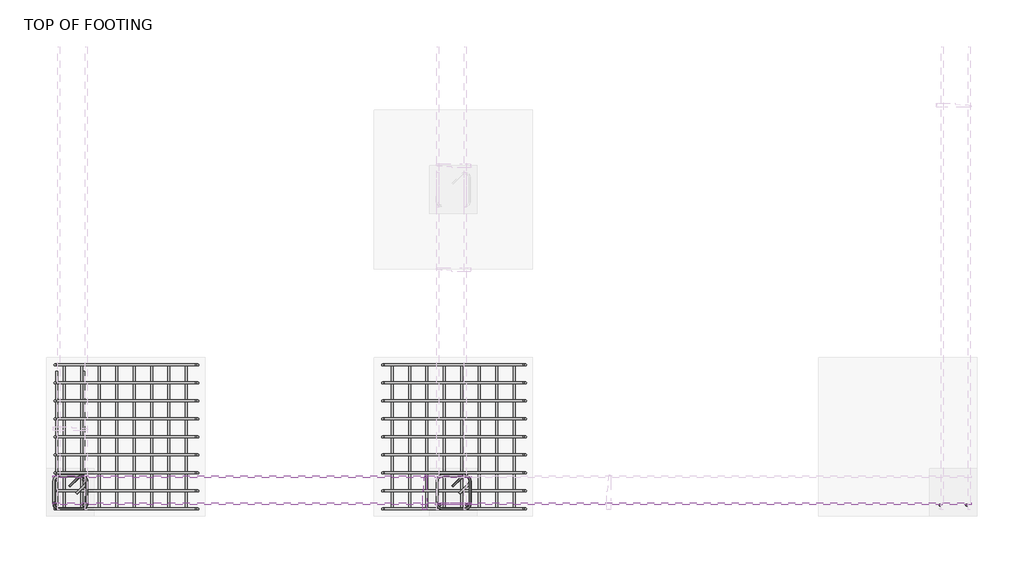
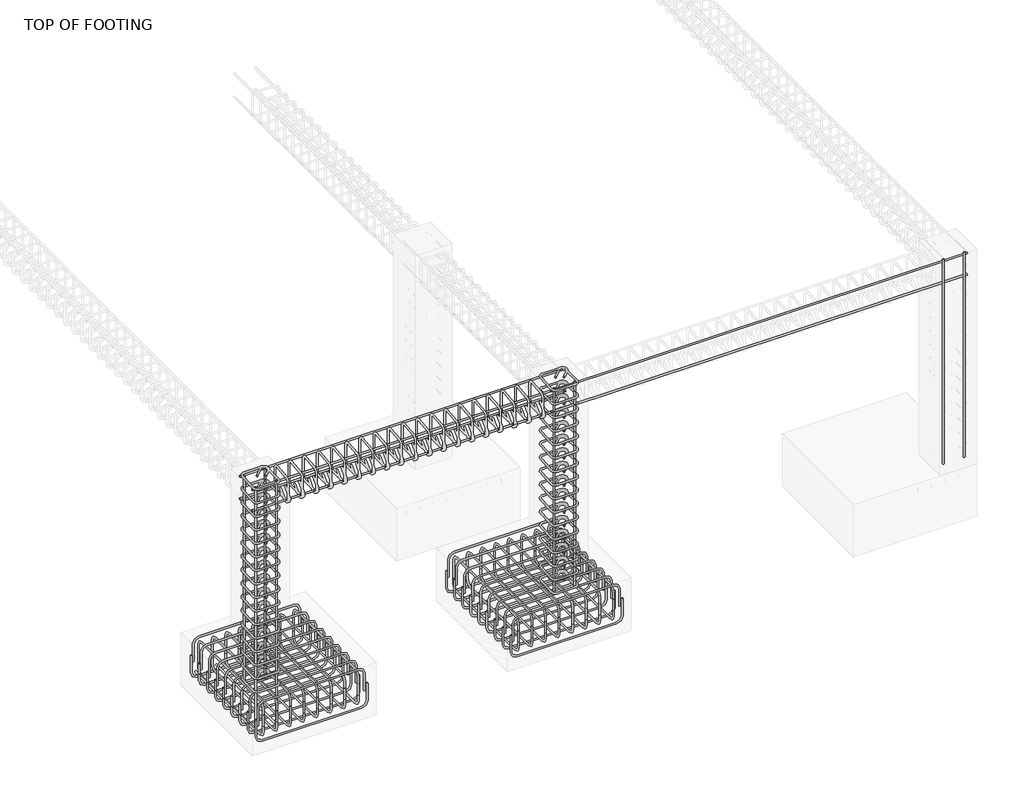
# One storey, part 2 of 10: 18 reinforcing bars.
"""IFC4 building model written with IfcOpenShell, lengths in millimetres."""

from ifc_helpers import new_model, si_unit, point, frame, origin, place, context, project, spatial, polyline, circle_curve, trimmed, segment, composite_curve, source, transform, mapped, element, save
from ifc_brep_helpers import swept_disk

model = new_model("IFC4")

# Units and contexts
model_context = context("Model", 3, world=origin())
ifc_project = project(units=[si_unit("LENGTHUNIT", "METRE", prefix="MILLI")], contexts=[model_context])

# Site, building, storey
site = spatial("IfcSite", under=ifc_project)
building = spatial("IfcBuilding", under=site)
storey = spatial("IfcBuildingStorey", under=building, Name="TOP OF FOOTING", Elevation=-1828.8)

# Reinforcing bars
placement = place(None, origin())
reinforcing_bar_shape = source(origin(), model_context, "Body", "SolidModel", [
    swept_disk(composite_curve([segment(polyline([(-9737.3957678, 8861.0767485, -2013.6880036), (-9737.3957678, 8861.0767485, -2160.9880036)]), True, "CONTINUOUS"), segment(trimmed(circle_curve(frame((-9783.7457678, 8861.0767485, -2160.9880036), z_axis=(0.0, 1.0, 0.0), x_axis=(46.349999999998545, 0.0, 0.0)), 46.35), [point((-9737.3957678, 8861.0767485, -2160.9880036))], [point((-9783.7457678, 8861.0767485, -2207.3380036))], True, "CARTESIAN"), True, "CONTINUOUS"), segment(polyline([(-9783.7457678, 8861.0767485, -2207.3380036), (-10591.4530437, 8861.0767485, -2207.3380036)]), True, "CONTINUOUS"), segment(trimmed(circle_curve(frame((-10591.4530437, 8861.0767485, -2160.9880036), z_axis=(0.0, 1.0, 0.0), x_axis=(0.0, 0.0, -46.34999999999991)), 46.35), [point((-10591.4530437, 8861.0767485, -2207.3380036))], [point((-10637.8030437, 8861.0767485, -2160.9880036))], True, "CARTESIAN"), True, "CONTINUOUS"), segment(polyline([(-10637.8030437, 8861.0767485, -2160.9880036), (-10637.8030437, 8861.0767485, -2013.6880036)]), True, "CONTINUOUS")], self_intersect=False), 6.35),
])
element("IfcReinforcingBar", 1, at=placement, inside=storey, context=model_context, shape_type="MappedRepresentation", body=[
    mapped(reinforcing_bar_shape, transform((0.0, 0.0, 0.0), x_axis=(1.0, 0.0, 0.0), y_axis=(0.0, 1.0, 0.0), z_axis=(0.0, 0.0, 1.0))),
    mapped(reinforcing_bar_shape, transform((0.0, -113.4125, 0.0), x_axis=(1.0, 0.0, 0.0), y_axis=(0.0, 1.0, 0.0), z_axis=(0.0, 0.0, 1.0))),
    mapped(reinforcing_bar_shape, transform((0.0, -226.825, 0.0), x_axis=(1.0, 0.0, 0.0), y_axis=(0.0, 1.0, 0.0), z_axis=(0.0, 0.0, 1.0))),
    mapped(reinforcing_bar_shape, transform((0.0, -340.2375, 0.0), x_axis=(1.0, 0.0, 0.0), y_axis=(0.0, 1.0, 0.0), z_axis=(0.0, 0.0, 1.0))),
    mapped(reinforcing_bar_shape, transform((0.0, -453.65, 0.0), x_axis=(1.0, 0.0, 0.0), y_axis=(0.0, 1.0, 0.0), z_axis=(0.0, 0.0, 1.0))),
    mapped(reinforcing_bar_shape, transform((0.0, -567.0625, 0.0), x_axis=(1.0, 0.0, 0.0), y_axis=(0.0, 1.0, 0.0), z_axis=(0.0, 0.0, 1.0))),
    mapped(reinforcing_bar_shape, transform((0.0, -680.475, 0.0), x_axis=(1.0, 0.0, 0.0), y_axis=(0.0, 1.0, 0.0), z_axis=(0.0, 0.0, 1.0))),
    mapped(reinforcing_bar_shape, transform((0.0, -793.8875, 0.0), x_axis=(1.0, 0.0, 0.0), y_axis=(0.0, 1.0, 0.0), z_axis=(0.0, 0.0, 1.0))),
    mapped(reinforcing_bar_shape, transform((0.0, -907.3, 0.0), x_axis=(1.0, 0.0, 0.0), y_axis=(0.0, 1.0, 0.0), z_axis=(0.0, 0.0, 1.0))),
])
reinforcing_bar_2_shape = source(origin(), model_context, "Body", "SolidModel", [
    swept_disk(composite_curve([segment(polyline([(-10621.5548549, 8861.0767485, -2068.7560969), (-10621.5548549, 8861.0767485, -1921.4560969)]), True, "CONTINUOUS"), segment(trimmed(circle_curve(frame((-10575.2048549, 8861.0767485, -1921.4560969), z_axis=(0.0, 1.0, 0.0), x_axis=(-46.350000000000364, 0.0, 0.0)), 46.35), [point((-10621.5548549, 8861.0767485, -1921.4560969))], [point((-10575.2048549, 8861.0767485, -1875.1060969))], True, "CARTESIAN"), True, "CONTINUOUS"), segment(polyline([(-10575.2048549, 8861.0767485, -1875.1060969), (-9806.8133686, 8861.0767485, -1875.1060969)]), True, "CONTINUOUS"), segment(trimmed(circle_curve(frame((-9806.8133686, 8861.0767485, -1921.4560969), z_axis=(0.0, 1.0, 0.0), x_axis=(0.0, 0.0, 46.34999999999991)), 46.35), [point((-9806.8133686, 8861.0767485, -1875.1060969))], [point((-9760.4633686, 8861.0767485, -1921.4560969))], True, "CARTESIAN"), True, "CONTINUOUS"), segment(polyline([(-9760.4633686, 8861.0767485, -1921.4560969), (-9760.4633686, 8861.0767485, -2068.7560969)]), True, "CONTINUOUS")], self_intersect=False), 6.35),
])
element("IfcReinforcingBar", 2, at=placement, inside=storey, context=model_context, shape_type="MappedRepresentation", body=[
    mapped(reinforcing_bar_2_shape, transform((0.0, 0.0, 0.0), x_axis=(1.0, 0.0, 0.0), y_axis=(0.0, 1.0, 0.0), z_axis=(0.0, 0.0, 1.0))),
    mapped(reinforcing_bar_2_shape, transform((0.0, -113.4125, 0.0), x_axis=(1.0, 0.0, 0.0), y_axis=(0.0, 1.0, 0.0), z_axis=(0.0, 0.0, 1.0))),
    mapped(reinforcing_bar_2_shape, transform((0.0, -226.825, 0.0), x_axis=(1.0, 0.0, 0.0), y_axis=(0.0, 1.0, 0.0), z_axis=(0.0, 0.0, 1.0))),
    mapped(reinforcing_bar_2_shape, transform((0.0, -340.2375, 0.0), x_axis=(1.0, 0.0, 0.0), y_axis=(0.0, 1.0, 0.0), z_axis=(0.0, 0.0, 1.0))),
    mapped(reinforcing_bar_2_shape, transform((0.0, -453.65, 0.0), x_axis=(1.0, 0.0, 0.0), y_axis=(0.0, 1.0, 0.0), z_axis=(0.0, 0.0, 1.0))),
    mapped(reinforcing_bar_2_shape, transform((0.0, -567.0625, 0.0), x_axis=(1.0, 0.0, 0.0), y_axis=(0.0, 1.0, 0.0), z_axis=(0.0, 0.0, 1.0))),
    mapped(reinforcing_bar_2_shape, transform((0.0, -680.475, 0.0), x_axis=(1.0, 0.0, 0.0), y_axis=(0.0, 1.0, 0.0), z_axis=(0.0, 0.0, 1.0))),
    mapped(reinforcing_bar_2_shape, transform((0.0, -793.8875, 0.0), x_axis=(1.0, 0.0, 0.0), y_axis=(0.0, 1.0, 0.0), z_axis=(0.0, 0.0, 1.0))),
    mapped(reinforcing_bar_2_shape, transform((0.0, -907.3, 0.0), x_axis=(1.0, 0.0, 0.0), y_axis=(0.0, 1.0, 0.0), z_axis=(0.0, 0.0, 1.0))),
])
reinforcing_bar_3_shape = source(origin(), model_context, "Body", "SolidModel", [
    swept_disk(composite_curve([segment(polyline([(-9809.6682872, 8861.0767485, -2087.4821199), (-9809.6682872, 8861.0767485, -1940.1821199)]), True, "CONTINUOUS"), segment(trimmed(circle_curve(frame((-9809.6682872, 8814.7267485, -1940.1821199), z_axis=(1.0, 0.0, 0.0), x_axis=(0.0, 46.350000000000364, 0.0)), 46.35), [point((-9809.6682872, 8861.0767485, -1940.1821199))], [point((-9809.6682872, 8814.7267485, -1893.8321199))], True, "CARTESIAN"), True, "CONTINUOUS"), segment(polyline([(-9809.6682872, 8814.7267485, -1893.8321199), (-9809.6682872, 8000.1267485, -1893.8321199)]), True, "CONTINUOUS"), segment(trimmed(circle_curve(frame((-9809.6682872, 8000.1267485, -1940.1821199), z_axis=(1.0, 0.0, 0.0), x_axis=(0.0, 0.0, 46.350000000000136)), 46.35), [point((-9809.6682872, 8000.1267485, -1893.8321199))], [point((-9809.6682872, 7953.7767485, -1940.1821199))], True, "CARTESIAN"), True, "CONTINUOUS"), segment(polyline([(-9809.6682872, 7953.7767485, -1940.1821199), (-9809.6682872, 7953.7767485, -2087.4821199)]), True, "CONTINUOUS")], self_intersect=False), 6.35),
])
element("IfcReinforcingBar", 3, at=placement, inside=storey, context=model_context, shape_type="MappedRepresentation", body=[
    mapped(reinforcing_bar_3_shape, transform((0.0, 0.0, 0.0), x_axis=(1.0, 0.0, 0.0), y_axis=(0.0, 1.0, 0.0), z_axis=(0.0, 0.0, 1.0))),
    mapped(reinforcing_bar_3_shape, transform((-109.824938, 0.0, 0.0), x_axis=(1.0, 0.0, 0.0), y_axis=(0.0, 1.0, 0.0), z_axis=(0.0, 0.0, 1.0))),
    mapped(reinforcing_bar_3_shape, transform((-219.649876, 0.0, 0.0), x_axis=(1.0, 0.0, 0.0), y_axis=(0.0, 1.0, 0.0), z_axis=(0.0, 0.0, 1.0))),
    mapped(reinforcing_bar_3_shape, transform((-329.474814, 0.0, 0.0), x_axis=(1.0, 0.0, 0.0), y_axis=(0.0, 1.0, 0.0), z_axis=(0.0, 0.0, 1.0))),
    mapped(reinforcing_bar_3_shape, transform((-439.299752, 0.0, 0.0), x_axis=(1.0, 0.0, 0.0), y_axis=(0.0, 1.0, 0.0), z_axis=(0.0, 0.0, 1.0))),
    mapped(reinforcing_bar_3_shape, transform((-549.12469, 0.0, 0.0), x_axis=(1.0, 0.0, 0.0), y_axis=(0.0, 1.0, 0.0), z_axis=(0.0, 0.0, 1.0))),
    mapped(reinforcing_bar_3_shape, transform((-658.949628, 0.0, 0.0), x_axis=(1.0, 0.0, 0.0), y_axis=(0.0, 1.0, 0.0), z_axis=(0.0, 0.0, 1.0))),
    mapped(reinforcing_bar_3_shape, transform((-768.774566, 0.0, 0.0), x_axis=(1.0, 0.0, 0.0), y_axis=(0.0, 1.0, 0.0), z_axis=(0.0, 0.0, 1.0))),
])
reinforcing_bar_4_shape = source(origin(), model_context, "Body", "SolidModel", [
    swept_disk(composite_curve([segment(polyline([(-10578.4428532, 8861.0767485, -1990.1985611), (-10578.4428532, 8861.0767485, -2137.4985611)]), True, "CONTINUOUS"), segment(trimmed(circle_curve(frame((-10578.4428532, 8814.7267485, -2137.4985611), z_axis=(-1.0, 0.0, 0.0), x_axis=(0.0, 46.350000000000364, 0.0)), 46.35), [point((-10578.4428532, 8861.0767485, -2137.4985611))], [point((-10578.4428532, 8814.7267485, -2183.8485611))], True, "CARTESIAN"), True, "CONTINUOUS"), segment(polyline([(-10578.4428532, 8814.7267485, -2183.8485611), (-10578.4428532, 8000.1267485, -2183.8485611)]), True, "CONTINUOUS"), segment(trimmed(circle_curve(frame((-10578.4428532, 8000.1267485, -2137.4985611), z_axis=(-1.0, 0.0, 0.0), x_axis=(0.0, 0.0, -46.34999999999991)), 46.35), [point((-10578.4428532, 8000.1267485, -2183.8485611))], [point((-10578.4428532, 7953.7767485, -2137.4985611))], True, "CARTESIAN"), True, "CONTINUOUS"), segment(polyline([(-10578.4428532, 7953.7767485, -2137.4985611), (-10578.4428532, 7953.7767485, -1990.1985611)]), True, "CONTINUOUS")], self_intersect=False), 6.35),
])
element("IfcReinforcingBar", 4, at=placement, inside=storey, context=model_context, shape_type="MappedRepresentation", body=[
    mapped(reinforcing_bar_4_shape, transform((0.0, 0.0, 0.0), x_axis=(1.0, 0.0, 0.0), y_axis=(0.0, 1.0, 0.0), z_axis=(0.0, 0.0, 1.0))),
    mapped(reinforcing_bar_4_shape, transform((109.824938, 0.0, 0.0), x_axis=(1.0, 0.0, 0.0), y_axis=(0.0, 1.0, 0.0), z_axis=(0.0, 0.0, 1.0))),
    mapped(reinforcing_bar_4_shape, transform((219.649876, 0.0, 0.0), x_axis=(1.0, 0.0, 0.0), y_axis=(0.0, 1.0, 0.0), z_axis=(0.0, 0.0, 1.0))),
    mapped(reinforcing_bar_4_shape, transform((329.474814, 0.0, 0.0), x_axis=(1.0, 0.0, 0.0), y_axis=(0.0, 1.0, 0.0), z_axis=(0.0, 0.0, 1.0))),
    mapped(reinforcing_bar_4_shape, transform((439.299752, 0.0, 0.0), x_axis=(1.0, 0.0, 0.0), y_axis=(0.0, 1.0, 0.0), z_axis=(0.0, 0.0, 1.0))),
    mapped(reinforcing_bar_4_shape, transform((549.12469, 0.0, 0.0), x_axis=(1.0, 0.0, 0.0), y_axis=(0.0, 1.0, 0.0), z_axis=(0.0, 0.0, 1.0))),
    mapped(reinforcing_bar_4_shape, transform((658.949628, 0.0, 0.0), x_axis=(1.0, 0.0, 0.0), y_axis=(0.0, 1.0, 0.0), z_axis=(0.0, 0.0, 1.0))),
    mapped(reinforcing_bar_4_shape, transform((768.774566, 0.0, 0.0), x_axis=(1.0, 0.0, 0.0), y_axis=(0.0, 1.0, 0.0), z_axis=(0.0, 0.0, 1.0))),
])
reinforcing_bar_5_shape = source(origin(), model_context, "Body", "SolidModel", [
    swept_disk(composite_curve([segment(polyline([(-7671.9957678, 8861.0767485, -2013.6880036), (-7671.9957678, 8861.0767485, -2160.9880036)]), True, "CONTINUOUS"), segment(trimmed(circle_curve(frame((-7718.3457678, 8861.0767485, -2160.9880036), z_axis=(0.0, 1.0, 0.0), x_axis=(46.350000000000364, 0.0, 0.0)), 46.35), [point((-7671.9957678, 8861.0767485, -2160.9880036))], [point((-7718.3457678, 8861.0767485, -2207.3380036))], True, "CARTESIAN"), True, "CONTINUOUS"), segment(polyline([(-7718.3457678, 8861.0767485, -2207.3380036), (-8526.0530437, 8861.0767485, -2207.3380036)]), True, "CONTINUOUS"), segment(trimmed(circle_curve(frame((-8526.0530437, 8861.0767485, -2160.9880036), z_axis=(0.0, 1.0, 0.0), x_axis=(0.0, 0.0, -46.34999999999991)), 46.35), [point((-8526.0530437, 8861.0767485, -2207.3380036))], [point((-8572.4030437, 8861.0767485, -2160.9880036))], True, "CARTESIAN"), True, "CONTINUOUS"), segment(polyline([(-8572.4030437, 8861.0767485, -2160.9880036), (-8572.4030437, 8861.0767485, -2013.6880036)]), True, "CONTINUOUS")], self_intersect=False), 6.35),
])
element("IfcReinforcingBar", 5, at=placement, inside=storey, context=model_context, shape_type="MappedRepresentation", body=[
    mapped(reinforcing_bar_5_shape, transform((0.0, 0.0, 0.0), x_axis=(1.0, 0.0, 0.0), y_axis=(0.0, 1.0, 0.0), z_axis=(0.0, 0.0, 1.0))),
    mapped(reinforcing_bar_5_shape, transform((0.0, -113.4125, 0.0), x_axis=(1.0, 0.0, 0.0), y_axis=(0.0, 1.0, 0.0), z_axis=(0.0, 0.0, 1.0))),
    mapped(reinforcing_bar_5_shape, transform((0.0, -226.825, 0.0), x_axis=(1.0, 0.0, 0.0), y_axis=(0.0, 1.0, 0.0), z_axis=(0.0, 0.0, 1.0))),
    mapped(reinforcing_bar_5_shape, transform((0.0, -340.2375, 0.0), x_axis=(1.0, 0.0, 0.0), y_axis=(0.0, 1.0, 0.0), z_axis=(0.0, 0.0, 1.0))),
    mapped(reinforcing_bar_5_shape, transform((0.0, -453.65, 0.0), x_axis=(1.0, 0.0, 0.0), y_axis=(0.0, 1.0, 0.0), z_axis=(0.0, 0.0, 1.0))),
    mapped(reinforcing_bar_5_shape, transform((0.0, -567.0625, 0.0), x_axis=(1.0, 0.0, 0.0), y_axis=(0.0, 1.0, 0.0), z_axis=(0.0, 0.0, 1.0))),
    mapped(reinforcing_bar_5_shape, transform((0.0, -680.475, 0.0), x_axis=(1.0, 0.0, 0.0), y_axis=(0.0, 1.0, 0.0), z_axis=(0.0, 0.0, 1.0))),
    mapped(reinforcing_bar_5_shape, transform((0.0, -793.8875, 0.0), x_axis=(1.0, 0.0, 0.0), y_axis=(0.0, 1.0, 0.0), z_axis=(0.0, 0.0, 1.0))),
    mapped(reinforcing_bar_5_shape, transform((0.0, -907.3, 0.0), x_axis=(1.0, 0.0, 0.0), y_axis=(0.0, 1.0, 0.0), z_axis=(0.0, 0.0, 1.0))),
])
reinforcing_bar_6_shape = source(origin(), model_context, "Body", "SolidModel", [
    swept_disk(composite_curve([segment(polyline([(-8556.1548549, 8861.0767485, -2068.7560969), (-8556.1548549, 8861.0767485, -1921.4560969)]), True, "CONTINUOUS"), segment(trimmed(circle_curve(frame((-8509.8048549, 8861.0767485, -1921.4560969), z_axis=(0.0, 1.0, 0.0), x_axis=(-46.350000000000364, 0.0, 0.0)), 46.35), [point((-8556.1548549, 8861.0767485, -1921.4560969))], [point((-8509.8048549, 8861.0767485, -1875.1060969))], True, "CARTESIAN"), True, "CONTINUOUS"), segment(polyline([(-8509.8048549, 8861.0767485, -1875.1060969), (-7741.4133686, 8861.0767485, -1875.1060969)]), True, "CONTINUOUS"), segment(trimmed(circle_curve(frame((-7741.4133686, 8861.0767485, -1921.4560969), z_axis=(0.0, 1.0, 0.0), x_axis=(0.0, 0.0, 46.34999999999991)), 46.35), [point((-7741.4133686, 8861.0767485, -1875.1060969))], [point((-7695.0633686, 8861.0767485, -1921.4560969))], True, "CARTESIAN"), True, "CONTINUOUS"), segment(polyline([(-7695.0633686, 8861.0767485, -1921.4560969), (-7695.0633686, 8861.0767485, -2068.7560969)]), True, "CONTINUOUS")], self_intersect=False), 6.35),
])
element("IfcReinforcingBar", 6, at=placement, inside=storey, context=model_context, shape_type="MappedRepresentation", body=[
    mapped(reinforcing_bar_6_shape, transform((0.0, 0.0, 0.0), x_axis=(1.0, 0.0, 0.0), y_axis=(0.0, 1.0, 0.0), z_axis=(0.0, 0.0, 1.0))),
    mapped(reinforcing_bar_6_shape, transform((0.0, -113.4125, 0.0), x_axis=(1.0, 0.0, 0.0), y_axis=(0.0, 1.0, 0.0), z_axis=(0.0, 0.0, 1.0))),
    mapped(reinforcing_bar_6_shape, transform((0.0, -226.825, 0.0), x_axis=(1.0, 0.0, 0.0), y_axis=(0.0, 1.0, 0.0), z_axis=(0.0, 0.0, 1.0))),
    mapped(reinforcing_bar_6_shape, transform((0.0, -340.2375, 0.0), x_axis=(1.0, 0.0, 0.0), y_axis=(0.0, 1.0, 0.0), z_axis=(0.0, 0.0, 1.0))),
    mapped(reinforcing_bar_6_shape, transform((0.0, -453.65, 0.0), x_axis=(1.0, 0.0, 0.0), y_axis=(0.0, 1.0, 0.0), z_axis=(0.0, 0.0, 1.0))),
    mapped(reinforcing_bar_6_shape, transform((0.0, -567.0625, 0.0), x_axis=(1.0, 0.0, 0.0), y_axis=(0.0, 1.0, 0.0), z_axis=(0.0, 0.0, 1.0))),
    mapped(reinforcing_bar_6_shape, transform((0.0, -680.475, 0.0), x_axis=(1.0, 0.0, 0.0), y_axis=(0.0, 1.0, 0.0), z_axis=(0.0, 0.0, 1.0))),
    mapped(reinforcing_bar_6_shape, transform((0.0, -793.8875, 0.0), x_axis=(1.0, 0.0, 0.0), y_axis=(0.0, 1.0, 0.0), z_axis=(0.0, 0.0, 1.0))),
    mapped(reinforcing_bar_6_shape, transform((0.0, -907.3, 0.0), x_axis=(1.0, 0.0, 0.0), y_axis=(0.0, 1.0, 0.0), z_axis=(0.0, 0.0, 1.0))),
])
reinforcing_bar_7_shape = source(origin(), model_context, "Body", "SolidModel", [
    swept_disk(composite_curve([segment(polyline([(-7744.2682872, 8861.0767485, -2087.4821199), (-7744.2682872, 8861.0767485, -1940.1821199)]), True, "CONTINUOUS"), segment(trimmed(circle_curve(frame((-7744.2682872, 8814.7267485, -1940.1821199), z_axis=(1.0, 0.0, 0.0), x_axis=(0.0, 46.350000000000364, 0.0)), 46.35), [point((-7744.2682872, 8861.0767485, -1940.1821199))], [point((-7744.2682872, 8814.7267485, -1893.8321199))], True, "CARTESIAN"), True, "CONTINUOUS"), segment(polyline([(-7744.2682872, 8814.7267485, -1893.8321199), (-7744.2682872, 8000.1267485, -1893.8321199)]), True, "CONTINUOUS"), segment(trimmed(circle_curve(frame((-7744.2682872, 8000.1267485, -1940.1821199), z_axis=(1.0, 0.0, 0.0), x_axis=(0.0, 0.0, 46.350000000000136)), 46.35), [point((-7744.2682872, 8000.1267485, -1893.8321199))], [point((-7744.2682872, 7953.7767485, -1940.1821199))], True, "CARTESIAN"), True, "CONTINUOUS"), segment(polyline([(-7744.2682872, 7953.7767485, -1940.1821199), (-7744.2682872, 7953.7767485, -2087.4821199)]), True, "CONTINUOUS")], self_intersect=False), 6.35),
])
element("IfcReinforcingBar", 7, at=placement, inside=storey, context=model_context, shape_type="MappedRepresentation", body=[
    mapped(reinforcing_bar_7_shape, transform((0.0, 0.0, 0.0), x_axis=(1.0, 0.0, 0.0), y_axis=(0.0, 1.0, 0.0), z_axis=(0.0, 0.0, 1.0))),
    mapped(reinforcing_bar_7_shape, transform((-109.824938, 0.0, 0.0), x_axis=(1.0, 0.0, 0.0), y_axis=(0.0, 1.0, 0.0), z_axis=(0.0, 0.0, 1.0))),
    mapped(reinforcing_bar_7_shape, transform((-219.649876, 0.0, 0.0), x_axis=(1.0, 0.0, 0.0), y_axis=(0.0, 1.0, 0.0), z_axis=(0.0, 0.0, 1.0))),
    mapped(reinforcing_bar_7_shape, transform((-329.474814, 0.0, 0.0), x_axis=(1.0, 0.0, 0.0), y_axis=(0.0, 1.0, 0.0), z_axis=(0.0, 0.0, 1.0))),
    mapped(reinforcing_bar_7_shape, transform((-439.299752, 0.0, 0.0), x_axis=(1.0, 0.0, 0.0), y_axis=(0.0, 1.0, 0.0), z_axis=(0.0, 0.0, 1.0))),
    mapped(reinforcing_bar_7_shape, transform((-549.12469, 0.0, 0.0), x_axis=(1.0, 0.0, 0.0), y_axis=(0.0, 1.0, 0.0), z_axis=(0.0, 0.0, 1.0))),
    mapped(reinforcing_bar_7_shape, transform((-658.949628, 0.0, 0.0), x_axis=(1.0, 0.0, 0.0), y_axis=(0.0, 1.0, 0.0), z_axis=(0.0, 0.0, 1.0))),
    mapped(reinforcing_bar_7_shape, transform((-768.774566, 0.0, 0.0), x_axis=(1.0, 0.0, 0.0), y_axis=(0.0, 1.0, 0.0), z_axis=(0.0, 0.0, 1.0))),
])
reinforcing_bar_8_shape = source(origin(), model_context, "Body", "SolidModel", [
    swept_disk(composite_curve([segment(polyline([(-8513.0428532, 8861.0767485, -1990.1985611), (-8513.0428532, 8861.0767485, -2137.4985611)]), True, "CONTINUOUS"), segment(trimmed(circle_curve(frame((-8513.0428532, 8814.7267485, -2137.4985611), z_axis=(-1.0, 0.0, 0.0), x_axis=(0.0, 46.350000000000364, 0.0)), 46.35), [point((-8513.0428532, 8861.0767485, -2137.4985611))], [point((-8513.0428532, 8814.7267485, -2183.8485611))], True, "CARTESIAN"), True, "CONTINUOUS"), segment(polyline([(-8513.0428532, 8814.7267485, -2183.8485611), (-8513.0428532, 8000.1267485, -2183.8485611)]), True, "CONTINUOUS"), segment(trimmed(circle_curve(frame((-8513.0428532, 8000.1267485, -2137.4985611), z_axis=(-1.0, 0.0, 0.0), x_axis=(0.0, 0.0, -46.34999999999991)), 46.35), [point((-8513.0428532, 8000.1267485, -2183.8485611))], [point((-8513.0428532, 7953.7767485, -2137.4985611))], True, "CARTESIAN"), True, "CONTINUOUS"), segment(polyline([(-8513.0428532, 7953.7767485, -2137.4985611), (-8513.0428532, 7953.7767485, -1990.1985611)]), True, "CONTINUOUS")], self_intersect=False), 6.35),
])
element("IfcReinforcingBar", 8, at=placement, inside=storey, context=model_context, shape_type="MappedRepresentation", body=[
    mapped(reinforcing_bar_8_shape, transform((0.0, 0.0, 0.0), x_axis=(1.0, 0.0, 0.0), y_axis=(0.0, 1.0, 0.0), z_axis=(0.0, 0.0, 1.0))),
    mapped(reinforcing_bar_8_shape, transform((109.824938, 0.0, 0.0), x_axis=(1.0, 0.0, 0.0), y_axis=(0.0, 1.0, 0.0), z_axis=(0.0, 0.0, 1.0))),
    mapped(reinforcing_bar_8_shape, transform((219.649876, 0.0, 0.0), x_axis=(1.0, 0.0, 0.0), y_axis=(0.0, 1.0, 0.0), z_axis=(0.0, 0.0, 1.0))),
    mapped(reinforcing_bar_8_shape, transform((329.474814, 0.0, 0.0), x_axis=(1.0, 0.0, 0.0), y_axis=(0.0, 1.0, 0.0), z_axis=(0.0, 0.0, 1.0))),
    mapped(reinforcing_bar_8_shape, transform((439.299752, 0.0, 0.0), x_axis=(1.0, 0.0, 0.0), y_axis=(0.0, 1.0, 0.0), z_axis=(0.0, 0.0, 1.0))),
    mapped(reinforcing_bar_8_shape, transform((549.12469, 0.0, 0.0), x_axis=(1.0, 0.0, 0.0), y_axis=(0.0, 1.0, 0.0), z_axis=(0.0, 0.0, 1.0))),
    mapped(reinforcing_bar_8_shape, transform((658.949628, 0.0, 0.0), x_axis=(1.0, 0.0, 0.0), y_axis=(0.0, 1.0, 0.0), z_axis=(0.0, 0.0, 1.0))),
    mapped(reinforcing_bar_8_shape, transform((768.774566, 0.0, 0.0), x_axis=(1.0, 0.0, 0.0), y_axis=(0.0, 1.0, 0.0), z_axis=(0.0, 0.0, 1.0))),
])
reinforcing_bar_9_shape = source(origin(), model_context, "Body", "SolidModel", [
    swept_disk(composite_curve([segment(polyline([(-4890.7163335, 7977.6267485, -1788.8), (-4890.7163335, 7977.6267485, -40.0)]), True, "CONTINUOUS")], self_intersect=False), 6.35),
])
element("IfcReinforcingBar", 9, at=placement, inside=storey, context=model_context, shape_type="MappedRepresentation", body=[
    mapped(reinforcing_bar_9_shape, transform((0.0, 0.0, 0.0), x_axis=(1.0, 0.0, 0.0), y_axis=(0.0, 1.0, 0.0), z_axis=(0.0, 0.0, 1.0))),
    mapped(reinforcing_bar_9_shape, transform((-168.8572682, 0.0, 0.0), x_axis=(1.0, 0.0, 0.0), y_axis=(0.0, 1.0, 0.0), z_axis=(0.0, 0.0, 1.0))),
])
reinforcing_bar_10_shape = source(origin(), model_context, "Body", "SolidModel", [
    swept_disk(composite_curve([segment(polyline([(-10546.6571284, 8096.1509831, -46.35), (-10490.9135654, 8151.8945461, -46.35)]), True, "CONTINUOUS"), segment(trimmed(circle_curve(frame((-10468.7457678, 8129.7267485, -46.35), z_axis=(0.0, 0.0, -1.0), x_axis=(-22.167797600000995, 22.167797600000085, 0.0)), 31.35), [point((-10490.9135654, 8151.8945461, -46.35))], [point((-10437.3957678, 8129.7267485, -46.35))], True, "CARTESIAN"), True, "CONTINUOUS"), segment(polyline([(-10437.3957678, 8129.7267485, -46.35), (-10437.3957678, 7985.1267485, -46.35)]), True, "CONTINUOUS"), segment(trimmed(circle_curve(frame((-10468.7457678, 7985.1267485, -46.35), z_axis=(0.0, 0.0, -1.0), x_axis=(31.349999999998545, 0.0, 0.0)), 31.35), [point((-10437.3957678, 7985.1267485, -46.35))], [point((-10468.7457678, 7953.7767485, -46.35))], True, "CARTESIAN"), True, "CONTINUOUS"), segment(polyline([(-10468.7457678, 7953.7767485, -46.35), (-10613.3457678, 7953.7767485, -46.35)]), True, "CONTINUOUS"), segment(trimmed(circle_curve(frame((-10613.3457678, 7985.0680812, -44.4329719), z_axis=(0.0, 0.06114922175001322, -0.9981286353368326), x_axis=(0.0, -31.291332699999657, -1.9170281000000031)), 31.35), [point((-10613.3457678, 7953.7767485, -46.35))], [point((-10644.6957678, 7985.0680812, -44.4329719))], True, "CARTESIAN"), True, "CONTINUOUS"), segment(polyline([(-10644.6957678, 7985.0680812, -44.4329719), (-10644.6957678, 8129.7854158, -35.5670281)]), True, "CONTINUOUS"), segment(trimmed(circle_curve(frame((-10613.3457678, 8129.7854158, -35.5670281), z_axis=(0.0, 0.06114922175001322, -0.9981286353368326), x_axis=(-31.350000000000364, 0.0, 0.0)), 31.35), [point((-10644.6957678, 8129.7854158, -35.5670281))], [point((-10613.3457678, 8161.0767485, -33.65))], True, "CARTESIAN"), True, "CONTINUOUS"), segment(polyline([(-10613.3457678, 8161.0767485, -33.65), (-10468.7457678, 8161.0767485, -33.65)]), True, "CONTINUOUS"), segment(trimmed(circle_curve(frame((-10468.7457678, 8129.7267485, -33.65), z_axis=(0.0, 0.0, -1.0), x_axis=(0.0, 31.349999999999454, 0.0)), 31.35), [point((-10468.7457678, 8161.0767485, -33.65))], [point((-10446.5779702, 8107.5589509, -33.65))], True, "CARTESIAN"), True, "CONTINUOUS"), segment(polyline([(-10446.5779702, 8107.5589509, -33.65), (-10502.3215332, 8051.8153879, -33.65)]), True, "CONTINUOUS")], self_intersect=False), 6.35),
])
element("IfcReinforcingBar", 10, at=placement, inside=storey, context=model_context, shape_type="MappedRepresentation", body=[
    mapped(reinforcing_bar_10_shape, transform((0.0, 0.0, 0.0), x_axis=(1.0, 0.0, 0.0), y_axis=(0.0, 1.0, 0.0), z_axis=(0.0, 0.0, 1.0))),
    mapped(reinforcing_bar_10_shape, transform((0.0, 0.0, -115.74), x_axis=(1.0, 0.0, 0.0), y_axis=(0.0, 1.0, 0.0), z_axis=(0.0, 0.0, 1.0))),
    mapped(reinforcing_bar_10_shape, transform((0.0, 0.0, -231.48), x_axis=(1.0, 0.0, 0.0), y_axis=(0.0, 1.0, 0.0), z_axis=(0.0, 0.0, 1.0))),
    mapped(reinforcing_bar_10_shape, transform((0.0, 0.0, -347.22), x_axis=(1.0, 0.0, 0.0), y_axis=(0.0, 1.0, 0.0), z_axis=(0.0, 0.0, 1.0))),
    mapped(reinforcing_bar_10_shape, transform((0.0, 0.0, -462.96), x_axis=(1.0, 0.0, 0.0), y_axis=(0.0, 1.0, 0.0), z_axis=(0.0, 0.0, 1.0))),
    mapped(reinforcing_bar_10_shape, transform((0.0, 0.0, -578.7), x_axis=(1.0, 0.0, 0.0), y_axis=(0.0, 1.0, 0.0), z_axis=(0.0, 0.0, 1.0))),
    mapped(reinforcing_bar_10_shape, transform((0.0, 0.0, -694.44), x_axis=(1.0, 0.0, 0.0), y_axis=(0.0, 1.0, 0.0), z_axis=(0.0, 0.0, 1.0))),
    mapped(reinforcing_bar_10_shape, transform((0.0, 0.0, -810.18), x_axis=(1.0, 0.0, 0.0), y_axis=(0.0, 1.0, 0.0), z_axis=(0.0, 0.0, 1.0))),
    mapped(reinforcing_bar_10_shape, transform((0.0, 0.0, -925.92), x_axis=(1.0, 0.0, 0.0), y_axis=(0.0, 1.0, 0.0), z_axis=(0.0, 0.0, 1.0))),
    mapped(reinforcing_bar_10_shape, transform((0.0, 0.0, -1041.66), x_axis=(1.0, 0.0, 0.0), y_axis=(0.0, 1.0, 0.0), z_axis=(0.0, 0.0, 1.0))),
    mapped(reinforcing_bar_10_shape, transform((0.0, 0.0, -1157.4), x_axis=(1.0, 0.0, 0.0), y_axis=(0.0, 1.0, 0.0), z_axis=(0.0, 0.0, 1.0))),
    mapped(reinforcing_bar_10_shape, transform((0.0, 0.0, -1273.14), x_axis=(1.0, 0.0, 0.0), y_axis=(0.0, 1.0, 0.0), z_axis=(0.0, 0.0, 1.0))),
    mapped(reinforcing_bar_10_shape, transform((0.0, 0.0, -1388.88), x_axis=(1.0, 0.0, 0.0), y_axis=(0.0, 1.0, 0.0), z_axis=(0.0, 0.0, 1.0))),
    mapped(reinforcing_bar_10_shape, transform((0.0, 0.0, -1504.62), x_axis=(1.0, 0.0, 0.0), y_axis=(0.0, 1.0, 0.0), z_axis=(0.0, 0.0, 1.0))),
    mapped(reinforcing_bar_10_shape, transform((0.0, 0.0, -1620.36), x_axis=(1.0, 0.0, 0.0), y_axis=(0.0, 1.0, 0.0), z_axis=(0.0, 0.0, 1.0))),
    mapped(reinforcing_bar_10_shape, transform((0.0, 0.0, -1736.1), x_axis=(1.0, 0.0, 0.0), y_axis=(0.0, 1.0, 0.0), z_axis=(0.0, 0.0, 1.0))),
])
reinforcing_bar_11_shape = source(origin(), model_context, "Body", "SolidModel", [
    swept_disk(composite_curve([segment(polyline([(-10458.1163335, 8137.2267485, -1788.8), (-10458.1163335, 8137.2267485, -40.0)]), True, "CONTINUOUS")], self_intersect=False), 6.35),
])
element("IfcReinforcingBar", 11, at=placement, inside=storey, context=model_context, shape_type="MappedRepresentation", body=[
    mapped(reinforcing_bar_11_shape, transform((0.0, 0.0, 0.0), x_axis=(1.0, 0.0, 0.0), y_axis=(0.0, 1.0, 0.0), z_axis=(0.0, 0.0, 1.0))),
    mapped(reinforcing_bar_11_shape, transform((-168.8572682, 0.0, 0.0), x_axis=(1.0, 0.0, 0.0), y_axis=(0.0, 1.0, 0.0), z_axis=(0.0, 0.0, 1.0))),
])
reinforcing_bar_12_shape = source(origin(), model_context, "Body", "SolidModel", [
    swept_disk(composite_curve([segment(polyline([(-10458.1163335, 8821.9578683, -2131.4311305), (-10458.1163335, 8023.9767485, -2131.4311305)]), True, "CONTINUOUS"), segment(trimmed(circle_curve(frame((-10458.1163335, 8023.9767485, -2085.0811305), z_axis=(-1.0, 0.0, 0.0), x_axis=(0.0, 0.0, -46.34999999999991)), 46.35), [point((-10458.1163335, 8023.9767485, -2131.4311305))], [point((-10458.1163335, 7977.6267485, -2085.0811305))], True, "CARTESIAN"), True, "CONTINUOUS"), segment(polyline([(-10458.1163335, 7977.6267485, -2085.0811305), (-10458.1163335, 7977.6267485, -40.0)]), True, "CONTINUOUS")], self_intersect=False), 6.35),
])
element("IfcReinforcingBar", 12, at=placement, inside=storey, context=model_context, shape_type="MappedRepresentation", body=[
    mapped(reinforcing_bar_12_shape, transform((0.0, 0.0, 0.0), x_axis=(1.0, 0.0, 0.0), y_axis=(0.0, 1.0, 0.0), z_axis=(0.0, 0.0, 1.0))),
    mapped(reinforcing_bar_12_shape, transform((-168.8572682, 0.0, 0.0), x_axis=(1.0, 0.0, 0.0), y_axis=(0.0, 1.0, 0.0), z_axis=(0.0, 0.0, 1.0))),
])
reinforcing_bar_13_shape = source(origin(), model_context, "Body", "SolidModel", [
    swept_disk(composite_curve([segment(polyline([(-8131.2571284, 8096.1509831, -46.35), (-8075.5135654, 8151.8945461, -46.35)]), True, "CONTINUOUS"), segment(trimmed(circle_curve(frame((-8053.3457678, 8129.7267485, -46.35), z_axis=(0.0, 0.0, -1.0), x_axis=(-22.167797599999176, 22.167797600000085, 0.0)), 31.35), [point((-8075.5135654, 8151.8945461, -46.35))], [point((-8021.9957678, 8129.7267485, -46.35))], True, "CARTESIAN"), True, "CONTINUOUS"), segment(polyline([(-8021.9957678, 8129.7267485, -46.35), (-8021.9957678, 7985.1267485, -46.35)]), True, "CONTINUOUS"), segment(trimmed(circle_curve(frame((-8053.3457678, 7985.1267485, -46.35), z_axis=(0.0, 0.0, -1.0), x_axis=(31.350000000000364, 0.0, 0.0)), 31.35), [point((-8021.9957678, 7985.1267485, -46.35))], [point((-8053.3457678, 7953.7767485, -46.35))], True, "CARTESIAN"), True, "CONTINUOUS"), segment(polyline([(-8053.3457678, 7953.7767485, -46.35), (-8197.9457678, 7953.7767485, -46.35)]), True, "CONTINUOUS"), segment(trimmed(circle_curve(frame((-8197.9457678, 7985.0680812, -44.4329719), z_axis=(0.0, 0.06114922175001322, -0.9981286353368326), x_axis=(0.0, -31.291332699999657, -1.9170281000000031)), 31.35), [point((-8197.9457678, 7953.7767485, -46.35))], [point((-8229.2957678, 7985.0680812, -44.4329719))], True, "CARTESIAN"), True, "CONTINUOUS"), segment(polyline([(-8229.2957678, 7985.0680812, -44.4329719), (-8229.2957678, 8129.7854158, -35.5670281)]), True, "CONTINUOUS"), segment(trimmed(circle_curve(frame((-8197.9457678, 8129.7854158, -35.5670281), z_axis=(0.0, 0.06114922175001322, -0.9981286353368326), x_axis=(-31.350000000000364, 0.0, 0.0)), 31.35), [point((-8229.2957678, 8129.7854158, -35.5670281))], [point((-8197.9457678, 8161.0767485, -33.65))], True, "CARTESIAN"), True, "CONTINUOUS"), segment(polyline([(-8197.9457678, 8161.0767485, -33.65), (-8053.3457678, 8161.0767485, -33.65)]), True, "CONTINUOUS"), segment(trimmed(circle_curve(frame((-8053.3457678, 8129.7267485, -33.65), z_axis=(0.0, 0.0, -1.0), x_axis=(0.0, 31.349999999999454, 0.0)), 31.35), [point((-8053.3457678, 8161.0767485, -33.65))], [point((-8031.1779702, 8107.5589509, -33.65))], True, "CARTESIAN"), True, "CONTINUOUS"), segment(polyline([(-8031.1779702, 8107.5589509, -33.65), (-8086.9215332, 8051.8153879, -33.65)]), True, "CONTINUOUS")], self_intersect=False), 6.35),
])
element("IfcReinforcingBar", 13, at=placement, inside=storey, context=model_context, shape_type="MappedRepresentation", body=[
    mapped(reinforcing_bar_13_shape, transform((0.0, 0.0, 0.0), x_axis=(1.0, 0.0, 0.0), y_axis=(0.0, 1.0, 0.0), z_axis=(0.0, 0.0, 1.0))),
    mapped(reinforcing_bar_13_shape, transform((0.0, 0.0, -115.74), x_axis=(1.0, 0.0, 0.0), y_axis=(0.0, 1.0, 0.0), z_axis=(0.0, 0.0, 1.0))),
    mapped(reinforcing_bar_13_shape, transform((0.0, 0.0, -231.48), x_axis=(1.0, 0.0, 0.0), y_axis=(0.0, 1.0, 0.0), z_axis=(0.0, 0.0, 1.0))),
    mapped(reinforcing_bar_13_shape, transform((0.0, 0.0, -347.22), x_axis=(1.0, 0.0, 0.0), y_axis=(0.0, 1.0, 0.0), z_axis=(0.0, 0.0, 1.0))),
    mapped(reinforcing_bar_13_shape, transform((0.0, 0.0, -462.96), x_axis=(1.0, 0.0, 0.0), y_axis=(0.0, 1.0, 0.0), z_axis=(0.0, 0.0, 1.0))),
    mapped(reinforcing_bar_13_shape, transform((0.0, 0.0, -578.7), x_axis=(1.0, 0.0, 0.0), y_axis=(0.0, 1.0, 0.0), z_axis=(0.0, 0.0, 1.0))),
    mapped(reinforcing_bar_13_shape, transform((0.0, 0.0, -694.44), x_axis=(1.0, 0.0, 0.0), y_axis=(0.0, 1.0, 0.0), z_axis=(0.0, 0.0, 1.0))),
    mapped(reinforcing_bar_13_shape, transform((0.0, 0.0, -810.18), x_axis=(1.0, 0.0, 0.0), y_axis=(0.0, 1.0, 0.0), z_axis=(0.0, 0.0, 1.0))),
    mapped(reinforcing_bar_13_shape, transform((0.0, 0.0, -925.92), x_axis=(1.0, 0.0, 0.0), y_axis=(0.0, 1.0, 0.0), z_axis=(0.0, 0.0, 1.0))),
    mapped(reinforcing_bar_13_shape, transform((0.0, 0.0, -1041.66), x_axis=(1.0, 0.0, 0.0), y_axis=(0.0, 1.0, 0.0), z_axis=(0.0, 0.0, 1.0))),
    mapped(reinforcing_bar_13_shape, transform((0.0, 0.0, -1157.4), x_axis=(1.0, 0.0, 0.0), y_axis=(0.0, 1.0, 0.0), z_axis=(0.0, 0.0, 1.0))),
    mapped(reinforcing_bar_13_shape, transform((0.0, 0.0, -1273.14), x_axis=(1.0, 0.0, 0.0), y_axis=(0.0, 1.0, 0.0), z_axis=(0.0, 0.0, 1.0))),
    mapped(reinforcing_bar_13_shape, transform((0.0, 0.0, -1388.88), x_axis=(1.0, 0.0, 0.0), y_axis=(0.0, 1.0, 0.0), z_axis=(0.0, 0.0, 1.0))),
    mapped(reinforcing_bar_13_shape, transform((0.0, 0.0, -1504.62), x_axis=(1.0, 0.0, 0.0), y_axis=(0.0, 1.0, 0.0), z_axis=(0.0, 0.0, 1.0))),
    mapped(reinforcing_bar_13_shape, transform((0.0, 0.0, -1620.36), x_axis=(1.0, 0.0, 0.0), y_axis=(0.0, 1.0, 0.0), z_axis=(0.0, 0.0, 1.0))),
    mapped(reinforcing_bar_13_shape, transform((0.0, 0.0, -1736.1), x_axis=(1.0, 0.0, 0.0), y_axis=(0.0, 1.0, 0.0), z_axis=(0.0, 0.0, 1.0))),
])
reinforcing_bar_14_shape = source(origin(), model_context, "Body", "SolidModel", [
    swept_disk(composite_curve([segment(polyline([(-8042.7163335, 7977.6267485, -1788.8), (-8042.7163335, 7977.6267485, -40.0)]), True, "CONTINUOUS")], self_intersect=False), 6.35),
])
element("IfcReinforcingBar", 14, at=placement, inside=storey, context=model_context, shape_type="MappedRepresentation", body=[
    mapped(reinforcing_bar_14_shape, transform((0.0, 0.0, 0.0), x_axis=(1.0, 0.0, 0.0), y_axis=(0.0, 1.0, 0.0), z_axis=(0.0, 0.0, 1.0))),
    mapped(reinforcing_bar_14_shape, transform((-168.8572682, 0.0, 0.0), x_axis=(1.0, 0.0, 0.0), y_axis=(0.0, 1.0, 0.0), z_axis=(0.0, 0.0, 1.0))),
])
reinforcing_bar_15_shape = source(origin(), model_context, "Body", "SolidModel", [
    swept_disk(composite_curve([segment(polyline([(-10364.6957678, 8018.7025138, -144.3886395), (-10364.6957678, 7962.9589509, -200.1322024)]), True, "CONTINUOUS"), segment(trimmed(circle_curve(frame((-10364.6957678, 7985.1267485, -222.3), z_axis=(1.0, 0.0, 0.0), x_axis=(0.0, -22.167797600000085, 22.1677976)), 31.35), [point((-10364.6957678, 7962.9589509, -200.1322024))], [point((-10364.6957678, 7985.1267485, -253.65))], True, "CARTESIAN"), True, "CONTINUOUS"), segment(polyline([(-10364.6957678, 7985.1267485, -253.65), (-10364.6957678, 8129.7267485, -253.65)]), True, "CONTINUOUS"), segment(trimmed(circle_curve(frame((-10364.6957678, 8129.7267485, -222.3), z_axis=(1.0, 0.0, 0.0), x_axis=(0.0, 0.0, -31.349999999999994)), 31.35), [point((-10364.6957678, 8129.7267485, -253.65))], [point((-10364.6957678, 8161.0767485, -222.3))], True, "CARTESIAN"), True, "CONTINUOUS"), segment(polyline([(-10364.6957678, 8161.0767485, -222.3), (-10364.6957678, 8161.0767485, -77.7)]), True, "CONTINUOUS"), segment(trimmed(circle_curve(frame((-10366.6127959, 8129.7854158, -77.7), z_axis=(0.9981286353368326, -0.06114922175001382, 0.0), x_axis=(1.917028100000607, 31.291332699999657, 0.0)), 31.35), [point((-10364.6957678, 8161.0767485, -77.7))], [point((-10366.6127959, 8129.7854158, -46.35))], True, "CARTESIAN"), True, "CONTINUOUS"), segment(polyline([(-10366.6127959, 8129.7854158, -46.35), (-10375.4787397, 7985.0680812, -46.35)]), True, "CONTINUOUS"), segment(trimmed(circle_curve(frame((-10375.4787397, 7985.0680812, -77.7), z_axis=(0.9981286353368326, -0.06114922175001382, 0.0), x_axis=(0.0, 0.0, 31.35)), 31.35), [point((-10375.4787397, 7985.0680812, -46.35))], [point((-10377.3957678, 7953.7767485, -77.7))], True, "CARTESIAN"), True, "CONTINUOUS"), segment(polyline([(-10377.3957678, 7953.7767485, -77.7), (-10377.3957678, 7953.7767485, -222.3)]), True, "CONTINUOUS"), segment(trimmed(circle_curve(frame((-10377.3957678, 7985.1267485, -222.3), z_axis=(1.0, 0.0, 0.0), x_axis=(0.0, -31.349999999999454, 0.0)), 31.35), [point((-10377.3957678, 7953.7767485, -222.3))], [point((-10377.3957678, 8007.2945461, -244.4677976))], True, "CARTESIAN"), True, "CONTINUOUS"), segment(polyline([(-10377.3957678, 8007.2945461, -244.4677976), (-10377.3957678, 8063.038109, -188.7242346)]), True, "CONTINUOUS")], self_intersect=False), 6.35),
])
element("IfcReinforcingBar", 15, at=placement, inside=storey, context=model_context, shape_type="MappedRepresentation", body=[
    mapped(reinforcing_bar_15_shape, transform((0.0, 0.0, 0.0), x_axis=(1.0, 0.0, 0.0), y_axis=(0.0, 1.0, 0.0), z_axis=(0.0, 0.0, 1.0))),
    mapped(reinforcing_bar_15_shape, transform((114.5944444, 0.0, 0.0), x_axis=(1.0, 0.0, 0.0), y_axis=(0.0, 1.0, 0.0), z_axis=(0.0, 0.0, 1.0))),
    mapped(reinforcing_bar_15_shape, transform((229.1888889, 0.0, 0.0), x_axis=(1.0, 0.0, 0.0), y_axis=(0.0, 1.0, 0.0), z_axis=(0.0, 0.0, 1.0))),
    mapped(reinforcing_bar_15_shape, transform((343.7833333, 0.0, 0.0), x_axis=(1.0, 0.0, 0.0), y_axis=(0.0, 1.0, 0.0), z_axis=(0.0, 0.0, 1.0))),
    mapped(reinforcing_bar_15_shape, transform((458.3777778, 0.0, 0.0), x_axis=(1.0, 0.0, 0.0), y_axis=(0.0, 1.0, 0.0), z_axis=(0.0, 0.0, 1.0))),
    mapped(reinforcing_bar_15_shape, transform((572.9722222, 0.0, 0.0), x_axis=(1.0, 0.0, 0.0), y_axis=(0.0, 1.0, 0.0), z_axis=(0.0, 0.0, 1.0))),
    mapped(reinforcing_bar_15_shape, transform((687.5666667, 0.0, 0.0), x_axis=(1.0, 0.0, 0.0), y_axis=(0.0, 1.0, 0.0), z_axis=(0.0, 0.0, 1.0))),
    mapped(reinforcing_bar_15_shape, transform((802.1611111, 0.0, 0.0), x_axis=(1.0, 0.0, 0.0), y_axis=(0.0, 1.0, 0.0), z_axis=(0.0, 0.0, 1.0))),
    mapped(reinforcing_bar_15_shape, transform((916.7555556, 0.0, 0.0), x_axis=(1.0, 0.0, 0.0), y_axis=(0.0, 1.0, 0.0), z_axis=(0.0, 0.0, 1.0))),
    mapped(reinforcing_bar_15_shape, transform((1031.35, 0.0, 0.0), x_axis=(1.0, 0.0, 0.0), y_axis=(0.0, 1.0, 0.0), z_axis=(0.0, 0.0, 1.0))),
    mapped(reinforcing_bar_15_shape, transform((1145.9444444, 0.0, 0.0), x_axis=(1.0, 0.0, 0.0), y_axis=(0.0, 1.0, 0.0), z_axis=(0.0, 0.0, 1.0))),
    mapped(reinforcing_bar_15_shape, transform((1260.5388889, 0.0, 0.0), x_axis=(1.0, 0.0, 0.0), y_axis=(0.0, 1.0, 0.0), z_axis=(0.0, 0.0, 1.0))),
    mapped(reinforcing_bar_15_shape, transform((1375.1333333, 0.0, 0.0), x_axis=(1.0, 0.0, 0.0), y_axis=(0.0, 1.0, 0.0), z_axis=(0.0, 0.0, 1.0))),
    mapped(reinforcing_bar_15_shape, transform((1489.7277778, 0.0, 0.0), x_axis=(1.0, 0.0, 0.0), y_axis=(0.0, 1.0, 0.0), z_axis=(0.0, 0.0, 1.0))),
    mapped(reinforcing_bar_15_shape, transform((1604.3222222, 0.0, 0.0), x_axis=(1.0, 0.0, 0.0), y_axis=(0.0, 1.0, 0.0), z_axis=(0.0, 0.0, 1.0))),
    mapped(reinforcing_bar_15_shape, transform((1718.9166667, 0.0, 0.0), x_axis=(1.0, 0.0, 0.0), y_axis=(0.0, 1.0, 0.0), z_axis=(0.0, 0.0, 1.0))),
    mapped(reinforcing_bar_15_shape, transform((1833.5111111, 0.0, 0.0), x_axis=(1.0, 0.0, 0.0), y_axis=(0.0, 1.0, 0.0), z_axis=(0.0, 0.0, 1.0))),
    mapped(reinforcing_bar_15_shape, transform((1948.1055556, 0.0, 0.0), x_axis=(1.0, 0.0, 0.0), y_axis=(0.0, 1.0, 0.0), z_axis=(0.0, 0.0, 1.0))),
    mapped(reinforcing_bar_15_shape, transform((2062.7, 0.0, 0.0), x_axis=(1.0, 0.0, 0.0), y_axis=(0.0, 1.0, 0.0), z_axis=(0.0, 0.0, 1.0))),
])
reinforcing_bar_16_shape = source(origin(), model_context, "Body", "SolidModel", [
    swept_disk(composite_curve([segment(polyline([(-10651.0457678, 7985.1267485, -240.95), (-8015.6457678, 7985.1267485, -240.95)]), True, "CONTINUOUS")], self_intersect=False), 6.35),
])
element("IfcReinforcingBar", 16, at=placement, inside=storey, context=model_context, shape_type="MappedRepresentation", body=[
    mapped(reinforcing_bar_16_shape, transform((0.0, 0.0, 0.0), x_axis=(1.0, 0.0, 0.0), y_axis=(0.0, 1.0, 0.0), z_axis=(0.0, 0.0, 1.0))),
    mapped(reinforcing_bar_16_shape, transform((0.0, 0.0, 181.9), x_axis=(1.0, 0.0, 0.0), y_axis=(0.0, 1.0, 0.0), z_axis=(0.0, 0.0, 1.0))),
])
reinforcing_bar_17_shape = source(origin(), model_context, "Body", "SolidModel", [
    swept_disk(composite_curve([segment(polyline([(-10651.0457678, 8156.7267485, -240.95), (-8015.6457678, 8156.7267485, -240.95)]), True, "CONTINUOUS")], self_intersect=False), 6.35),
])
element("IfcReinforcingBar", 17, at=placement, inside=storey, context=model_context, shape_type="MappedRepresentation", body=[
    mapped(reinforcing_bar_17_shape, transform((0.0, 0.0, 0.0), x_axis=(1.0, 0.0, 0.0), y_axis=(0.0, 1.0, 0.0), z_axis=(0.0, 0.0, 1.0))),
    mapped(reinforcing_bar_17_shape, transform((0.0, 0.0, 192.8258048), x_axis=(1.0, 0.0, 0.0), y_axis=(0.0, 1.0, 0.0), z_axis=(0.0, 0.0, 1.0))),
])
reinforcing_bar_18_shape = source(origin(), model_context, "Body", "SolidModel", [
    swept_disk(composite_curve([segment(polyline([(-8235.6457678, 7985.1267485, -240.95), (-4863.6457678, 7985.1267485, -240.95)]), True, "CONTINUOUS")], self_intersect=False), 6.35),
])
element("IfcReinforcingBar", 18, at=placement, inside=storey, context=model_context, shape_type="MappedRepresentation", body=[
    mapped(reinforcing_bar_18_shape, transform((0.0, 0.0, 0.0), x_axis=(1.0, 0.0, 0.0), y_axis=(0.0, 1.0, 0.0), z_axis=(0.0, 0.0, 1.0))),
    mapped(reinforcing_bar_18_shape, transform((0.0, 0.0, 181.9), x_axis=(1.0, 0.0, 0.0), y_axis=(0.0, 1.0, 0.0), z_axis=(0.0, 0.0, 1.0))),
])

save(model, "model.ifc")

# Revit data of these elements
# Elements 1, 2, 3, 4, 5, 6, 7, 8, 9, 10, 11, 12, 13, 14, 15, 16, 17, 18 (IfcReinforcingBar)
#   Phase Created = New Construction
